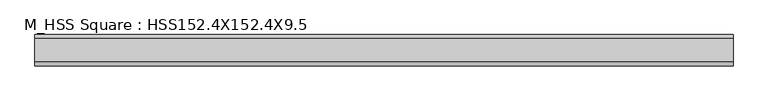
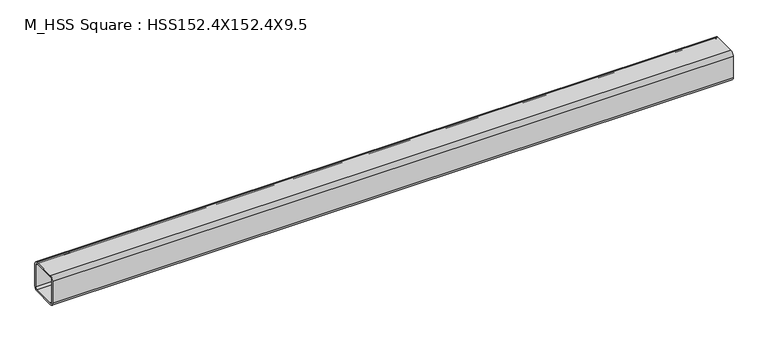
"""IFC4 building model written with IfcOpenShell, lengths in millimetres: beam geometry, M_HSS Square : HSS152.4X152.4X9.5."""

from ifc_helpers import new_model, si_unit, point, frame, frame_2d, origin, place, context, project, spatial, polyline, circle_curve, trimmed, segment, composite_curve, outline, extrude, source, transform, mapped, element, save


def m_hss_square_hss152_4x152_4x9_5_4d3a2309(model_context):
    return source(origin(), model_context, "Body", "SweptSolid", [
        extrude(outline(composite_curve([segment(trimmed(circle_curve(frame_2d((-56.94, 56.94)), 19.06), [point((-76.0, 56.94))], [point((-56.94, 76.0))], False, "CARTESIAN"), True, "CONTINUOUS"), segment(polyline([(-56.94, 76.0), (56.94, 76.0)]), True, "CONTINUOUS"), segment(trimmed(circle_curve(frame_2d((56.94, 56.94)), 19.06), [point((56.94, 76.0))], [point((76.0, 56.94))], False, "CARTESIAN"), True, "CONTINUOUS"), segment(polyline([(76.0, 56.94), (76.0, -56.94)]), True, "CONTINUOUS"), segment(trimmed(circle_curve(frame_2d((56.94, -56.94)), 19.06), [point((76.0, -56.94))], [point((56.94, -76.0))], False, "CARTESIAN"), True, "CONTINUOUS"), segment(polyline([(56.94, -76.0), (-56.94, -76.0)]), True, "CONTINUOUS"), segment(trimmed(circle_curve(frame_2d((-56.94, -56.94)), 19.06), [point((-56.94, -76.0))], [point((-76.0, -56.94))], False, "CARTESIAN"), True, "CONTINUOUS"), segment(polyline([(-76.0, -56.94), (-76.0, 56.94)]), True, "CONTINUOUS")], self_intersect=False), holes=[composite_curve([segment(polyline([(56.94, 66.47), (-56.94, 66.47)]), True, "CONTINUOUS"), segment(trimmed(circle_curve(frame_2d((-56.94, 56.94)), 9.53), [point((-56.94, 66.47))], [point((-66.47, 56.94))], True, "CARTESIAN"), True, "CONTINUOUS"), segment(polyline([(-66.47, 56.94), (-66.47, -56.94)]), True, "CONTINUOUS"), segment(trimmed(circle_curve(frame_2d((-56.94, -56.94)), 9.53), [point((-66.47, -56.94))], [point((-56.94, -66.47))], True, "CARTESIAN"), True, "CONTINUOUS"), segment(polyline([(-56.94, -66.47), (56.94, -66.47)]), True, "CONTINUOUS"), segment(trimmed(circle_curve(frame_2d((56.94, -56.94)), 9.53), [point((56.94, -66.47))], [point((66.47, -56.94))], True, "CARTESIAN"), True, "CONTINUOUS"), segment(polyline([(66.47, -56.94), (66.47, 56.94)]), True, "CONTINUOUS"), segment(trimmed(circle_curve(frame_2d((56.94, 56.94)), 9.53), [point((66.47, 56.94))], [point((56.94, 66.47))], True, "CARTESIAN"), True, "CONTINUOUS")], self_intersect=False)]), frame((-1737.2, 0.0, 0.0), z_axis=(1.0, 0.0, 0.0), x_axis=(0.0, 1.0, 0.0)), (0.0, 0.0, 1.0), 3374.5),
    ])


if __name__ == "__main__":
    model = new_model("IFC4")
    model_context = context("Model", 3, world=origin())
    ifc_project = project(units=[si_unit("LENGTHUNIT", "METRE", prefix="MILLI")], contexts=[model_context])
    site = spatial("IfcSite", under=ifc_project)
    building = spatial("IfcBuilding", under=site)
    placement = place(None, origin())
    m_hss_square_hss152_4x152_4x9_5_shape = m_hss_square_hss152_4x152_4x9_5_4d3a2309(model_context)
    element("IfcBeam", 1, ObjectType="M_HSS Square : HSS152.4X152.4X9.5", at=placement, inside=building, context=model_context, shape_type="MappedRepresentation", body=[
        mapped(m_hss_square_hss152_4x152_4x9_5_shape, transform((0.0, 0.0, 0.0), x_axis=(1.0, 0.0, 0.0), y_axis=(0.0, 1.0, 0.0), z_axis=(0.0, 0.0, 1.0))),
    ])
    save(model, "model.ifc")

# Revit data of these elements
# Type "M_HSS Square : HSS152.4X152.4X9.5"
#   Section Name Key = "HSS152.4X152.4X9.5"
#   Width = 15.2 cm
#   Wall Nominal Thickness = 0.953 cm
#   Wall Design Thickness = 0.886 cm
#   Torsional Moment of Inertia = 2690.00 cm⁴
#   Torsional Modulus = 362.0 cm³
#   Section Area = 48.9 cm²
#   Plastic Modulus weak axis = 259.0 cm³
#   Plastic Modulus strong axis = 259.0 cm³
#   Perimeter = 0.575 m²/m
#   Outer Fillet = 1.906 cm
#   Nominal Weight = 40.80 kgf/m
#   Moment of Inertia weak axis = 1640.00 cm⁴
#   Moment of Inertia strong axis = 1640.00 cm⁴
#   Length [instance default] = 5' - 0"
#   Inner Fillet = 0.953 cm
#   Height = 15.2 cm
#   Elastic Modulus weak axis = 216.0 cm³
#   Elastic Modulus strong axis = 216.0 cm³
#   Centroid Vertical = 7.6 cm
#   Centroid Horizontal = 7.6 cm
#   Structural Material [instance default] = Steel ASTM A500, Grade C, Rectangular and Square
# Element 1 (IfcBeam, "M_HSS Square : HSS152.4X152.4X9.5")
#   Structural Material = Metal - Steel 43-275
#   Materials on its faces: "Metal - Steel 43-275"
# Materials
#   "Steel ASTM A500, Grade C, Rectangular and Square": class "Metal", colour RGB 120 120 120, transparency 0, Description = "Carbon steel", Cost = 0
#   "Metal - Steel 43-275": class "Metal", colour RGB 247 247 247, transparency 0, Cost = 0
